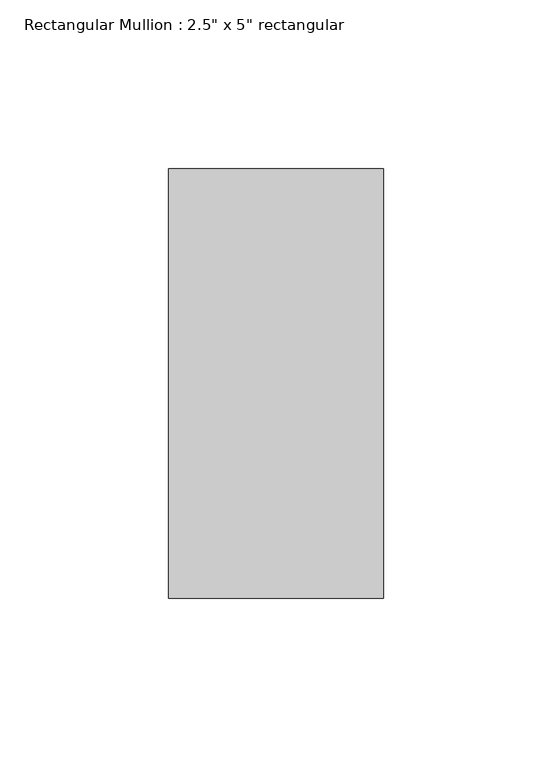
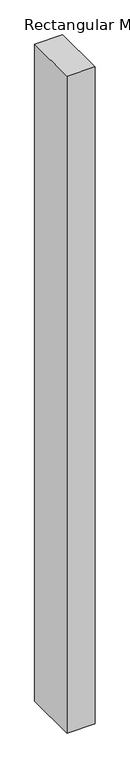
"""IFC4 building model written with IfcOpenShell, lengths in millimetres: member geometry."""

from ifc_helpers import new_model, si_unit, frame, origin, place, context, project, spatial, polyline, outline, extrude, source, transform, mapped, element, save


def member_44c1c08d(model_context):
    return source(origin(), model_context, "Body", "SweptSolid", [
        extrude(outline(polyline([(31.75, 63.5), (31.75, -63.5), (-31.75, -63.5), (-31.75, 63.5), (31.75, 63.5)])), frame((0.0, 0.0, -1578.2793787), z_axis=(0.0, 0.0, 1.0), x_axis=(1.0, 0.0, 0.0)), (0.0, 0.0, 1.0), 1578.2793787),
    ])


if __name__ == "__main__":
    model = new_model("IFC4")
    model_context = context("Model", 3, world=origin())
    ifc_project = project(units=[si_unit("LENGTHUNIT", "METRE", prefix="MILLI")], contexts=[model_context])
    site = spatial("IfcSite", under=ifc_project)
    building = spatial("IfcBuilding", under=site)
    placement = place(None, origin())
    member_shape = member_44c1c08d(model_context)
    element("IfcMember", 1, ObjectType="Rectangular Mullion : 2.5\" x 5\" rectangular", at=placement, inside=building, context=model_context, shape_type="MappedRepresentation", body=[
        mapped(member_shape, transform((0.0, 0.0, 0.0), x_axis=(1.0, 0.0, 0.0), y_axis=(0.0, 1.0, 0.0), z_axis=(0.0, 0.0, 1.0))),
    ])
    save(model, "model.ifc")

# Revit data of these elements
# Type "Rectangular Mullion : 2.5\" x 5\" rectangular"
#   built-in parameter 1007304 = 0.416667 (stored number, unit not read)
#   built-in parameter 1007301 = 0.104167 (stored number, unit not read)
#   built-in parameter 1007300 = 0.104167 (stored number, unit not read)
# Element 1 (IfcMember, "Rectangular Mullion : 2.5\" x 5\" rectangular")
#   Materials on its faces: "Aluminum"
# Materials
#   "Aluminum": class "Metal", colour RGB 247 247 247, transparency 0, Description = "Aluminum 6061", Cost = 0
